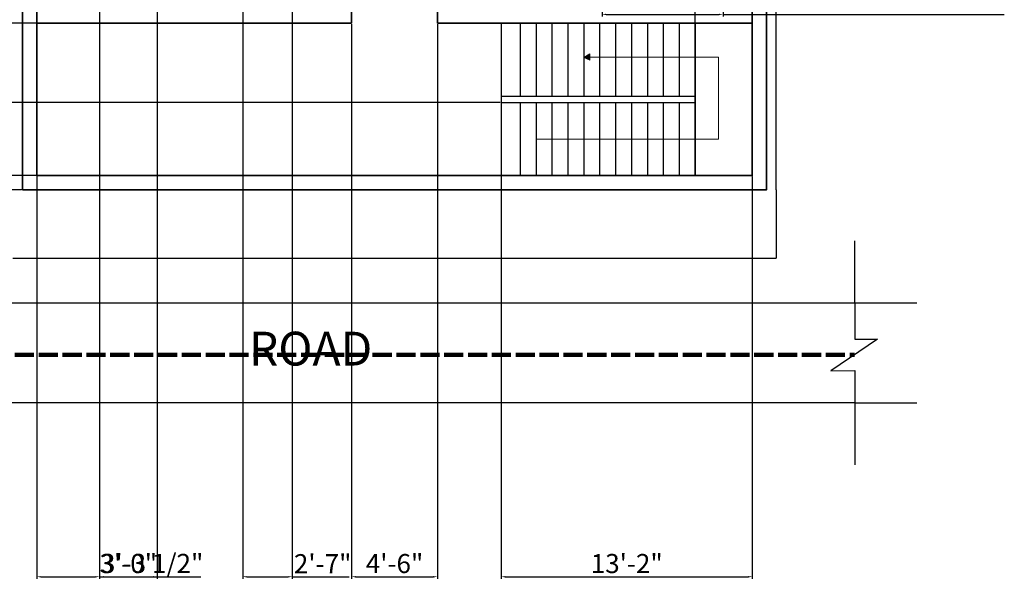
# Model space of a CAD drawing. Units: inches. Extents: x 1947 to 2903, y 1974 to 3472.
# Tile 2 of 5: x 2267 to 2887, y 1974 to 2335. Entities that reach past the tile are written whole.
import ezdxf

# ---------------------------------------------------------------- set-up
doc = ezdxf.new("R2010")
doc.units = ezdxf.units.IN
doc.linetypes.add('ACAD_ISO02W100', pattern=[15, 12, -3])
for name, color, linetype, lineweight in [('A-ANNO-DIMS', 2, 'Continuous', 18), ('A-ANNO-PATT', 7, 'Continuous', 13), ('A-ANNO-SYMB', 7, 'Continuous', 18), ('A-ANNO-TEXT', 7, 'Continuous', 18), ('A-FLOR-STRS', 7, 'Continuous', 25), ('A-WALL', 7, 'Continuous', 35), ('C-PROP', 1, 'Continuous', 25), ('C-ROAD', 7, 'Continuous', 25), ('C-ROAD-CNTR', 2, 'ACAD_ISO02W100', 100)]:
    doc.layers.add(name, color=color, linetype=linetype, lineweight=lineweight)
doc.styles.get("Standard").update_dxf_attribs({"font": 'arial.ttf'})
doc.dimstyles.new('ISO-25', dxfattribs={"dimtxt": 12, "dimasz": 2.5, "dimexe": 1.25, "dimexo": 0.625, "dimtad": 1, "dimdec": 0, "dimlunit": 4, "dimtxsty": 'Standard', "dimcen": 2.5, "dimadec": 0, "dimazin": 0, "dimtfac": 1, "dimtdec": 0, "dimtmove": 0, "dimatfit": 3, "dimfxl": 1, "dimarcsym": 0})

# ---------------------------------------------------------------- blocks, each defined once
blk = doc.blocks.new('*D6')
at = {"layer": 'A-ANNO-DIMS', "color": 0, "lineweight": -2, "transparency": 16777216}
for p, q in [((2268.49, 3341.41), (2191.31, 3341.41)), ((2192.56, 3338.91), (2192.56, 2230.91)), ((2268.49, 2228.41), (2191.31, 2228.41))]:
    blk.add_line(p, q, dxfattribs=at)
at = {"layer": 'A-ANNO-DIMS', "color": 0, "lineweight": 100, "transparency": 16777216}
for points in [[(2192.15, 3338.91), (2192.98, 3338.91), (2192.56, 3341.41)], [(2192.15, 2230.91), (2192.98, 2230.91), (2192.56, 2228.41)]]:
    blk.add_solid(points, dxfattribs=at)
at = {"layer": 'Defpoints', "color": 0, "lineweight": 100, "transparency": 16777216}
for p in [(2269.11, 3341.41), (2192.56, 2228.41), (2269.11, 2228.41)]:
    blk.add_point(p, dxfattribs=at)
at = {"layer": 'A-ANNO-DIMS', "color": 0, "transparency": 16777216, "insert": (2185.81, 2784.91), "char_height": 12, "attachment_point": 5, "rotation": 90}
blk.add_mtext('92\'-9"', dxfattribs=at)
blk = doc.blocks.new('*D21')
at = {"layer": 'A-ANNO-DIMS', "color": 0, "lineweight": -2, "transparency": 16777216}
for p, q in [((2633.63, 2349.59), (2633.63, 2337.56)), ((2709.7, 2349.59), (2709.7, 2337.56)), ((2636.13, 2338.81), (2707.2, 2338.81)), ((2709.7, 2338.81), (2886.59, 2338.81))]:
    blk.add_line(p, q, dxfattribs=at)
at = {"layer": 'A-ANNO-DIMS', "color": 0, "lineweight": 100, "transparency": 16777216}
for points in [[(2636.13, 2339.22), (2636.13, 2338.39), (2633.63, 2338.81)], [(2707.2, 2339.22), (2707.2, 2338.39), (2709.7, 2338.81)]]:
    blk.add_solid(points, dxfattribs=at)
at = {"layer": 'Defpoints', "color": 0, "lineweight": 100, "transparency": 16777216}
for p in [(2633.63, 2350.22), (2709.7, 2350.22), (2709.7, 2338.81)]:
    blk.add_point(p, dxfattribs=at)
at = {"layer": 'A-ANNO-DIMS', "color": 0, "transparency": 16777216, "insert": (2799.39, 2345.64), "char_height": 12, "attachment_point": 5}
blk.add_mtext('DINING SET 6\'-4" TYP.', dxfattribs=at)
blk = doc.blocks.new('*D33')
at = {"layer": 'A-ANNO-DIMS', "color": 0, "lineweight": -2, "transparency": 16777216}
for p, q in [((2476.11, 2332.59), (2476.11, 1983.7)), ((2530.11, 2332.59), (2530.11, 1983.7)), ((2478.61, 1984.95), (2527.61, 1984.95))]:
    blk.add_line(p, q, dxfattribs=at)
at = {"layer": 'A-ANNO-DIMS', "color": 0, "lineweight": 100, "transparency": 16777216}
for points in [[(2478.61, 1985.36), (2478.61, 1984.53), (2476.11, 1984.95)], [(2527.61, 1985.36), (2527.61, 1984.53), (2530.11, 1984.95)]]:
    blk.add_solid(points, dxfattribs=at)
at = {"layer": 'Defpoints', "color": 0, "lineweight": 100, "transparency": 16777216}
for p in [(2476.11, 2333.22), (2530.11, 2333.22), (2530.11, 1984.95)]:
    blk.add_point(p, dxfattribs=at)
at = {"layer": 'A-ANNO-DIMS', "color": 0, "transparency": 16777216, "insert": (2503.11, 1991.7), "char_height": 12, "attachment_point": 5}
blk.add_mtext('4\'-6"', dxfattribs=at)
blk = doc.blocks.new('*D34')
at = {"layer": 'A-ANNO-DIMS', "color": 0, "lineweight": -2, "transparency": 16777216}
for p, q in [((2268.49, 2228.41), (1970.32, 2228.41)), ((1971.57, 2225.91), (1971.57, 2187.91)), ((2262.49, 2185.41), (1970.32, 2185.41))]:
    blk.add_line(p, q, dxfattribs=at)
at = {"layer": 'A-ANNO-DIMS', "color": 0, "lineweight": 100, "transparency": 16777216}
for points in [[(1971.16, 2225.91), (1971.99, 2225.91), (1971.57, 2228.41)], [(1971.16, 2187.91), (1971.99, 2187.91), (1971.57, 2185.41)]]:
    blk.add_solid(points, dxfattribs=at)
at = {"layer": 'Defpoints', "color": 0, "lineweight": 100, "transparency": 16777216}
for p in [(2269.11, 2228.41), (1971.57, 2185.41), (2263.11, 2185.41)]:
    blk.add_point(p, dxfattribs=at)
at = {"layer": 'A-ANNO-DIMS', "color": 0, "transparency": 16777216, "insert": (1964.82, 2206.91), "char_height": 12, "attachment_point": 5, "rotation": 90}
blk.add_mtext('3\'-7"', dxfattribs=at)
blk = doc.blocks.new('*D35')
at = {"layer": 'A-ANNO-DIMS', "color": 0, "lineweight": -2, "transparency": 16777216}
for p, q in [((2277.49, 2333.22), (1970.32, 2333.22)), ((1971.57, 2239.91), (1971.57, 2330.72)), ((2277.49, 2237.41), (1970.32, 2237.41))]:
    blk.add_line(p, q, dxfattribs=at)
at = {"layer": 'A-ANNO-DIMS', "color": 0, "lineweight": 100, "transparency": 16777216}
for points in [[(1971.16, 2330.72), (1971.99, 2330.72), (1971.57, 2333.22)], [(1971.16, 2239.91), (1971.99, 2239.91), (1971.57, 2237.41)]]:
    blk.add_solid(points, dxfattribs=at)
at = {"layer": 'Defpoints', "color": 0, "lineweight": 100, "transparency": 16777216}
for p in [(1971.57, 2333.22), (2278.11, 2333.22), (2278.11, 2237.41)]:
    blk.add_point(p, dxfattribs=at)
at = {"layer": 'A-ANNO-DIMS', "color": 0, "transparency": 16777216, "insert": (1964.82, 2285.31), "char_height": 12, "attachment_point": 5, "rotation": 90}
blk.add_mtext('8\'-0"', dxfattribs=at)
blk = doc.blocks.new('*D36')
at = {"layer": 'A-ANNO-DIMS', "color": 0, "lineweight": -2, "transparency": 16777216}
for p, q in [((2692.11, 2238.03), (2692.11, 3458.67)), ((2694.61, 3457.42), (2725.61, 3457.42)), ((2728.11, 2238.03), (2728.11, 3458.67))]:
    blk.add_line(p, q, dxfattribs=at)
at = {"layer": 'A-ANNO-DIMS', "color": 0, "lineweight": 100, "transparency": 16777216}
for points in [[(2694.61, 3457.83), (2694.61, 3457), (2692.11, 3457.42)], [(2725.61, 3457.83), (2725.61, 3457), (2728.11, 3457.42)]]:
    blk.add_solid(points, dxfattribs=at)
at = {"layer": 'Defpoints', "color": 0, "lineweight": 100, "transparency": 16777216}
for p in [(2728.11, 3457.42), (2692.11, 2237.41), (2728.11, 2237.41)]:
    blk.add_point(p, dxfattribs=at)
at = {"layer": 'A-ANNO-DIMS', "color": 0, "transparency": 16777216, "insert": (2710.11, 3464.17), "char_height": 12, "attachment_point": 5}
blk.add_mtext('3\'-0"', dxfattribs=at)
blk = doc.blocks.new('*D37')
at = {"layer": 'A-ANNO-DIMS', "color": 0, "lineweight": -2, "transparency": 16777216}
for p, q in [((2570.2, 2236.78), (2570.2, 1983.7)), ((2728.11, 2236.78), (2728.11, 1983.7)), ((2572.7, 1984.95), (2725.61, 1984.95))]:
    blk.add_line(p, q, dxfattribs=at)
at = {"layer": 'A-ANNO-DIMS', "color": 0, "lineweight": 100, "transparency": 16777216}
for points in [[(2572.7, 1985.36), (2572.7, 1984.53), (2570.2, 1984.95)], [(2725.61, 1985.36), (2725.61, 1984.53), (2728.11, 1984.95)]]:
    blk.add_solid(points, dxfattribs=at)
at = {"layer": 'Defpoints', "color": 0, "lineweight": 100, "transparency": 16777216}
for p in [(2570.2, 2237.41), (2728.11, 2237.41), (2728.11, 1984.95)]:
    blk.add_point(p, dxfattribs=at)
at = {"layer": 'A-ANNO-DIMS', "color": 0, "transparency": 16777216, "insert": (2649.15, 1991.7), "char_height": 12, "attachment_point": 5}
blk.add_mtext('13\'-2"', dxfattribs=at)
blk = doc.blocks.new('*D41')
at = {"layer": 'A-ANNO-DIMS', "color": 0, "lineweight": -2, "transparency": 16777216}
for p, q in [((2407.63, 2461.27), (2407.63, 1983.7)), ((2438.73, 2461.27), (2438.73, 1983.7)), ((2410.13, 1984.95), (2436.23, 1984.95)), ((2438.73, 1984.95), (2474.58, 1984.95))]:
    blk.add_line(p, q, dxfattribs=at)
at = {"layer": 'A-ANNO-DIMS', "color": 0, "lineweight": 100, "transparency": 16777216}
for points in [[(2410.13, 1985.36), (2410.13, 1984.53), (2407.63, 1984.95)], [(2436.23, 1985.36), (2436.23, 1984.53), (2438.73, 1984.95)]]:
    blk.add_solid(points, dxfattribs=at)
at = {"layer": 'Defpoints', "color": 0, "lineweight": 100, "transparency": 16777216}
for p in [(2407.63, 2461.89), (2438.73, 2461.89), (2438.73, 1984.95)]:
    blk.add_point(p, dxfattribs=at)
at = {"layer": 'A-ANNO-DIMS', "color": 0, "transparency": 16777216, "insert": (2457.91, 1991.6), "char_height": 12, "attachment_point": 5}
blk.add_mtext('2\'-7"', dxfattribs=at)
blk = doc.blocks.new('*D42')
at = {"layer": 'A-ANNO-DIMS', "color": 0, "lineweight": -2, "transparency": 16777216}
for p, q in [((2317.62, 2461.59), (2317.62, 1983.7)), ((2353.75, 2461.59), (2353.75, 1983.7)), ((2320.12, 1984.95), (2351.25, 1984.95))]:
    blk.add_line(p, q, dxfattribs=at)
at = {"layer": 'A-ANNO-DIMS', "color": 0, "lineweight": 100, "transparency": 16777216}
for points in [[(2320.12, 1985.36), (2320.12, 1984.53), (2317.62, 1984.95)], [(2351.25, 1985.36), (2351.25, 1984.53), (2353.75, 1984.95)]]:
    blk.add_solid(points, dxfattribs=at)
at = {"layer": 'Defpoints', "color": 0, "lineweight": 100, "transparency": 16777216}
for p in [(2317.62, 2462.22), (2353.75, 2462.22), (2353.75, 1984.95)]:
    blk.add_point(p, dxfattribs=at)
at = {"layer": 'A-ANNO-DIMS', "color": 0, "transparency": 16777216, "insert": (2335.68, 1991.7), "char_height": 12, "attachment_point": 5}
blk.add_mtext('3\'-0"', dxfattribs=at)
blk = doc.blocks.new('*D44')
at = {"layer": 'A-ANNO-DIMS', "color": 0, "lineweight": -2, "transparency": 16777216}
for p, q in [((2569.57, 2283.31), (1970.32, 2283.31)), ((1971.57, 2239.91), (1971.57, 2280.81)), ((2569.57, 2237.41), (1970.32, 2237.41))]:
    blk.add_line(p, q, dxfattribs=at)
at = {"layer": 'A-ANNO-DIMS', "color": 0, "lineweight": 100, "transparency": 16777216}
for points in [[(1971.16, 2280.81), (1971.99, 2280.81), (1971.57, 2283.31)], [(1971.16, 2239.91), (1971.99, 2239.91), (1971.57, 2237.41)]]:
    blk.add_solid(points, dxfattribs=at)
at = {"layer": 'Defpoints', "color": 0, "lineweight": 100, "transparency": 16777216}
for p in [(1971.57, 2283.31), (2570.2, 2283.31), (2570.2, 2237.41)]:
    blk.add_point(p, dxfattribs=at)
at = {"layer": 'A-ANNO-DIMS', "color": 0, "transparency": 16777216, "insert": (1964.82, 2260.36), "char_height": 12, "attachment_point": 5, "rotation": 90}
blk.add_mtext('3\'-10"', dxfattribs=at)
blk = doc.blocks.new('*D46')
at = {"layer": 'A-ANNO-DIMS', "color": 0, "lineweight": -2, "transparency": 16777216}
for p, q in [((2278.11, 2461.59), (2278.11, 1983.7)), ((2317.62, 2461.59), (2317.62, 1983.7)), ((2280.61, 1984.95), (2315.12, 1984.95)), ((2317.62, 1984.95), (2381.22, 1984.95))]:
    blk.add_line(p, q, dxfattribs=at)
at = {"layer": 'A-ANNO-DIMS', "color": 0, "lineweight": 100, "transparency": 16777216}
for points in [[(2280.61, 1985.36), (2280.61, 1984.53), (2278.11, 1984.95)], [(2315.12, 1985.36), (2315.12, 1984.53), (2317.62, 1984.95)]]:
    blk.add_solid(points, dxfattribs=at)
at = {"layer": 'Defpoints', "color": 0, "lineweight": 100, "transparency": 16777216}
for p in [(2278.11, 2462.22), (2317.62, 2462.22), (2317.62, 1984.95)]:
    blk.add_point(p, dxfattribs=at)
at = {"layer": 'A-ANNO-DIMS', "color": 0, "transparency": 16777216, "insert": (2350.67, 1991.78), "char_height": 12, "attachment_point": 5}
blk.add_mtext('3\'-3 1/2"', dxfattribs=at)

msp = doc.modelspace()

# ---------------------------------------------------------------- hatches: boundary and pattern name
at = {"layer": 'A-ANNO-PATT'}
h = msp.add_hatch(color=256, dxfattribs=at)
h.dxf.hatch_style = 1
h.paths.add_polyline_path([(2626, 2313.89), (2622.11, 2311.75), (2626, 2309.89), (2626, 2311.89)])

# ---------------------------------------------------------------- linework, layer by layer
at = {"layer": 'A-ANNO-SYMB'}
for p, q in [((2626, 2313.89), (2622.11, 2311.75)), ((2622.11, 2311.75), (2626, 2309.89)), ((2626, 2311.89), (2626, 2313.89)), ((2706.88, 2311.89), (2626, 2311.89)), ((2626, 2311.89), (2626, 2309.89)), ((2626, 2309.89), (2626, 2311.89)), ((2706.88, 2260.36), (2706.88, 2311.89)), ((2592.11, 2260.36), (2706.88, 2260.36))]:
    msp.add_line(p, q, dxfattribs=at)
at = {"layer": 'A-FLOR-STRS'}
for p, q in [((2570.2, 2333.22), (2570.2, 2237.41)), ((2582.11, 2333.22), (2582.11, 2287.31)), ((2592.11, 2333.22), (2592.11, 2287.31)), ((2602.11, 2333.22), (2602.11, 2287.31)), ((2612.11, 2333.22), (2612.11, 2287.31)), ((2622.11, 2333.22), (2622.11, 2287.31)), ((2632.11, 2333.22), (2632.11, 2287.31)), ((2642.11, 2333.22), (2642.11, 2287.31)), ((2652.11, 2333.22), (2652.11, 2287.31)), ((2662.11, 2333.22), (2662.11, 2287.31)), ((2672.11, 2333.22), (2672.11, 2287.31)), ((2682.11, 2333.22), (2682.11, 2287.31)), ((2692.11, 2333.22), (2692.11, 2237.41)), ((2570.2, 2287.31), (2692.11, 2287.31)), ((2570.2, 2283.31), (2692.11, 2283.31)), ((2582.11, 2283.31), (2582.11, 2237.41)), ((2592.11, 2283.31), (2592.11, 2237.41)), ((2602.11, 2283.31), (2602.11, 2237.41)), ((2612.11, 2283.31), (2612.11, 2237.41)), ((2622.11, 2283.31), (2622.11, 2237.41)), ((2632.11, 2283.31), (2632.11, 2237.41)), ((2642.11, 2283.31), (2642.11, 2237.41)), ((2652.11, 2283.31), (2652.11, 2237.41)), ((2662.11, 2283.31), (2662.11, 2237.41)), ((2672.11, 2283.31), (2672.11, 2237.41)), ((2682.11, 2283.31), (2682.11, 2237.41))]:
    msp.add_line(p, q, dxfattribs=at)
at = {"layer": 'A-WALL'}
for p, q in [((2476.11, 2347), (2476.11, 2333.22)), ((2530.11, 2348.13), (2530.11, 2333.22)), ((2728.11, 2347), (2728.11, 2333.22)), ((2278.11, 2333.22), (2476.11, 2333.22)), ((2530.11, 2333.22), (2728.11, 2333.22)), ((2728.11, 2333.22), (2692.11, 2333.22))]:
    msp.add_line(p, q, dxfattribs=at)
for points in [[(2269.11, 2228.41), (2737.11, 2228.41), (2737.11, 3341.41), (2269.11, 3341.41)], [(2278.11, 2237.41), (2728.11, 2237.41), (2728.11, 3332.41), (2278.11, 3332.41)]]:
    msp.add_lwpolyline(points, close=True, dxfattribs=at)
at = {"layer": 'C-PROP'}
for p, q in [((2743.11, 2228.41), (2743.11, 3341.41)), ((2743.11, 2228.41), (2743.11, 2185.41)), ((2263.11, 2185.41), (2743.11, 2185.41))]:
    msp.add_line(p, q, dxfattribs=at)
at = {"layer": 'C-ROAD'}
for p, q in [((2792.52, 2157.31), (2792.52, 2196.31)), ((2792.52, 2157.31), (2831.52, 2157.31)), ((2806.82, 2134.53), (2777.53, 2114.51)), ((2792.52, 2134.53), (2806.82, 2134.53)), ((2777.53, 2114.51), (2792.52, 2114.81)), ((2792.52, 2094.4), (2792.52, 2055.4)), ((2792.52, 2094.4), (2831.52, 2094.4))]:
    msp.add_line(p, q, dxfattribs=at)
for points in [[(2081.02, 2132.17), (2081.02, 2157.31), (2792.52, 2157.31), (2792.52, 2134.53)], [(2792.52, 2114.81), (2792.52, 2094.4), (2081.02, 2094.4), (2081.02, 2112.46)]]:
    msp.add_lwpolyline(points, dxfattribs=at)
at = {"layer": 'C-ROAD-CNTR'}
msp.add_line((2084.35, 2124.67), (2792.4, 2124.67), dxfattribs=at)

# ---------------------------------------------------------------- texts
at = {"layer": 'A-ANNO-TEXT', "insert": (2411.58, 2139.11), "char_height": 21.263, "attachment_point": 1}
msp.add_mtext_dynamic_manual_height_columns('ROAD', width=169.0859, gutter_width=106.32, heights=[0], dxfattribs=at)

# ---------------------------------------------------------------- dimensions: what is measured, and where the dimension line sits
at = {"layer": 'A-ANNO-DIMS'}
for base, p1, p2, picture, middle in [((2728.11, 3457.42), (2692.11, 2237.41), (2728.11, 2237.41), '*D36', (2710.11, 3464.17)), ((2317.62, 1984.95), (2278.11, 2462.22), (2317.62, 2462.22), '*D46', (2350.67, 1991.78)), ((2353.75, 1984.95), (2317.62, 2462.22), (2353.75, 2462.22), '*D42', (2335.68, 1991.7)), ((2438.73, 1984.95), (2407.63, 2461.89), (2438.73, 2461.89), '*D41', (2457.91, 1991.6)), ((2530.11, 1984.95), (2476.11, 2333.22), (2530.11, 2333.22), '*D33', (2503.11, 1991.7)), ((2728.11, 1984.95), (2570.2, 2237.41), (2728.11, 2237.41), '*D37', (2649.15, 1991.7))]:
    dim = msp.add_linear_dim(base=base, p1=p1, p2=p2, dimstyle='ISO-25', override={"dimdec": 1, "dimlfac": 1, "dimrnd": 0, "dimzin": 1, "dimdsep": 46, "dimlunit": 4, "dimfrac": 2}, dxfattribs=at)
    dim.commit()
    dim.dimension.update_dxf_attribs({"geometry": picture, "text_midpoint": middle})
for base, p1, p2, override, picture, middle in [((2192.56, 2228.41), (2269.11, 3341.41), (2269.11, 2228.41), {"dimclrd": 0, "dimclre": 0, "dimclrt": 0}, '*D6', (2185.81, 2784.91)), ((1971.57, 2333.22), (2278.11, 2237.41), (2278.11, 2333.22), {"dimdec": 1, "dimlfac": 1, "dimrnd": 0, "dimzin": 1, "dimdsep": 46, "dimlunit": 4, "dimfrac": 2}, '*D35', (1964.82, 2285.31)), ((1971.57, 2283.31), (2570.2, 2237.41), (2570.2, 2283.31), {"dimdec": 1, "dimlfac": 1, "dimrnd": 0, "dimzin": 1, "dimdsep": 46, "dimlunit": 4, "dimfrac": 2}, '*D44', (1964.82, 2260.36)), ((1971.57, 2185.41), (2269.11, 2228.41), (2263.11, 2185.41), {"dimdec": 1, "dimlfac": 1, "dimrnd": 0, "dimzin": 1, "dimdsep": 46, "dimlunit": 4, "dimfrac": 2}, '*D34', (1964.82, 2206.91))]:
    dim = msp.add_linear_dim(base=base, p1=p1, p2=p2, angle=90, dimstyle='ISO-25', override=override, dxfattribs=at)
    dim.commit()
    dim.dimension.update_dxf_attribs({"geometry": picture, "text_midpoint": middle})
dim = msp.add_linear_dim(base=(2709.7, 2338.81), p1=(2633.63, 2350.22), p2=(2709.7, 2350.22), text='DINING SET <> TYP.', dimstyle='ISO-25', override={"dimdec": 1, "dimlfac": 1, "dimrnd": 0, "dimzin": 1, "dimdsep": 46, "dimlunit": 4, "dimfrac": 2}, dxfattribs=at)
dim.commit()
dim.dimension.update_dxf_attribs({"geometry": '*D21', "text_midpoint": (2799.39, 2345.64)})

doc.saveas('drawing.dxf')
